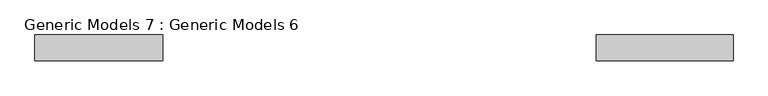
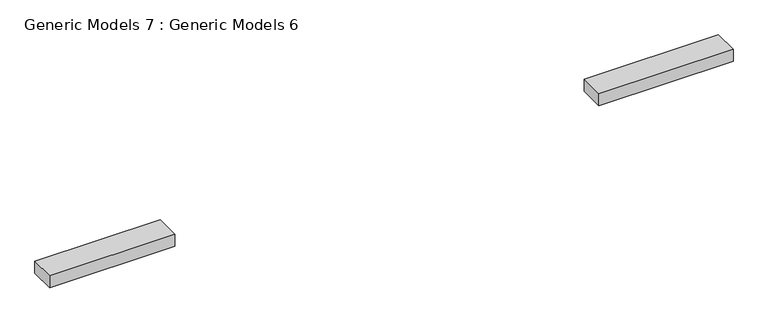
"""IFC4 building model written with IfcOpenShell, lengths in millimetres: proxy geometry, Generic Models 7 : Generic Models 6."""

from ifc_helpers import new_model, si_unit, frame, origin, place, context, project, spatial, polyline, outline, extrude, source, transform, mapped, element, save


def generic_models_7_generic_models_6_617e5b9e(model_context):
    return source(origin(), model_context, "Body", "SweptSolid", [
        extrude(outline(polyline([(-13705.2201591, 7039.4500875), (-12199.3157907, 7039.4500875), (-12199.3157907, 6734.6500875), (-13705.2201591, 6734.6500875), (-13705.2201591, 7039.4500875)])), frame((0.0, 0.0, 2133.6), z_axis=(0.0, 0.0, 1.0), x_axis=(1.0, 0.0, 0.0)), (0.0, 0.0, 1.0), 152.4),
        extrude(outline(polyline([(-7094.3452422, 7039.4500875), (-5480.7032006, 7039.4500875), (-5480.7032006, 6734.6500875), (-7094.3452422, 6734.6500875), (-7094.3452422, 7039.4500875)])), frame((0.0, 0.0, 2133.6), z_axis=(0.0, 0.0, 1.0), x_axis=(1.0, 0.0, 0.0)), (0.0, 0.0, 1.0), 152.4),
    ])


if __name__ == "__main__":
    model = new_model("IFC4")
    model_context = context("Model", 3, world=origin())
    ifc_project = project(units=[si_unit("LENGTHUNIT", "METRE", prefix="MILLI")], contexts=[model_context])
    site = spatial("IfcSite", under=ifc_project)
    building = spatial("IfcBuilding", under=site)
    placement = place(None, origin())
    generic_models_7_generic_models_6_shape = generic_models_7_generic_models_6_617e5b9e(model_context)
    element("IfcBuildingElementProxy", 1, Name="Generic Models 7 : Generic Models 6", ObjectType="Generic Models 7 : Generic Models 6", at=placement, inside=building, context=model_context, shape_type="MappedRepresentation", body=[
        mapped(generic_models_7_generic_models_6_shape, transform((0.0, 0.0, 0.0), x_axis=(1.0, 0.0, 0.0), y_axis=(0.0, 1.0, 0.0), z_axis=(0.0, 0.0, 1.0))),
    ])
    save(model, "model.ifc")

# Revit data of these elements
# Element 1 (IfcBuildingElementProxy, "Generic Models 7 : Generic Models 6")
#   Materials on its faces: "LIGHT BEIGE"
# Materials
#   "LIGHT BEIGE": class "Generic", colour RGB 120 120 120, transparency 0, Cost = 0
